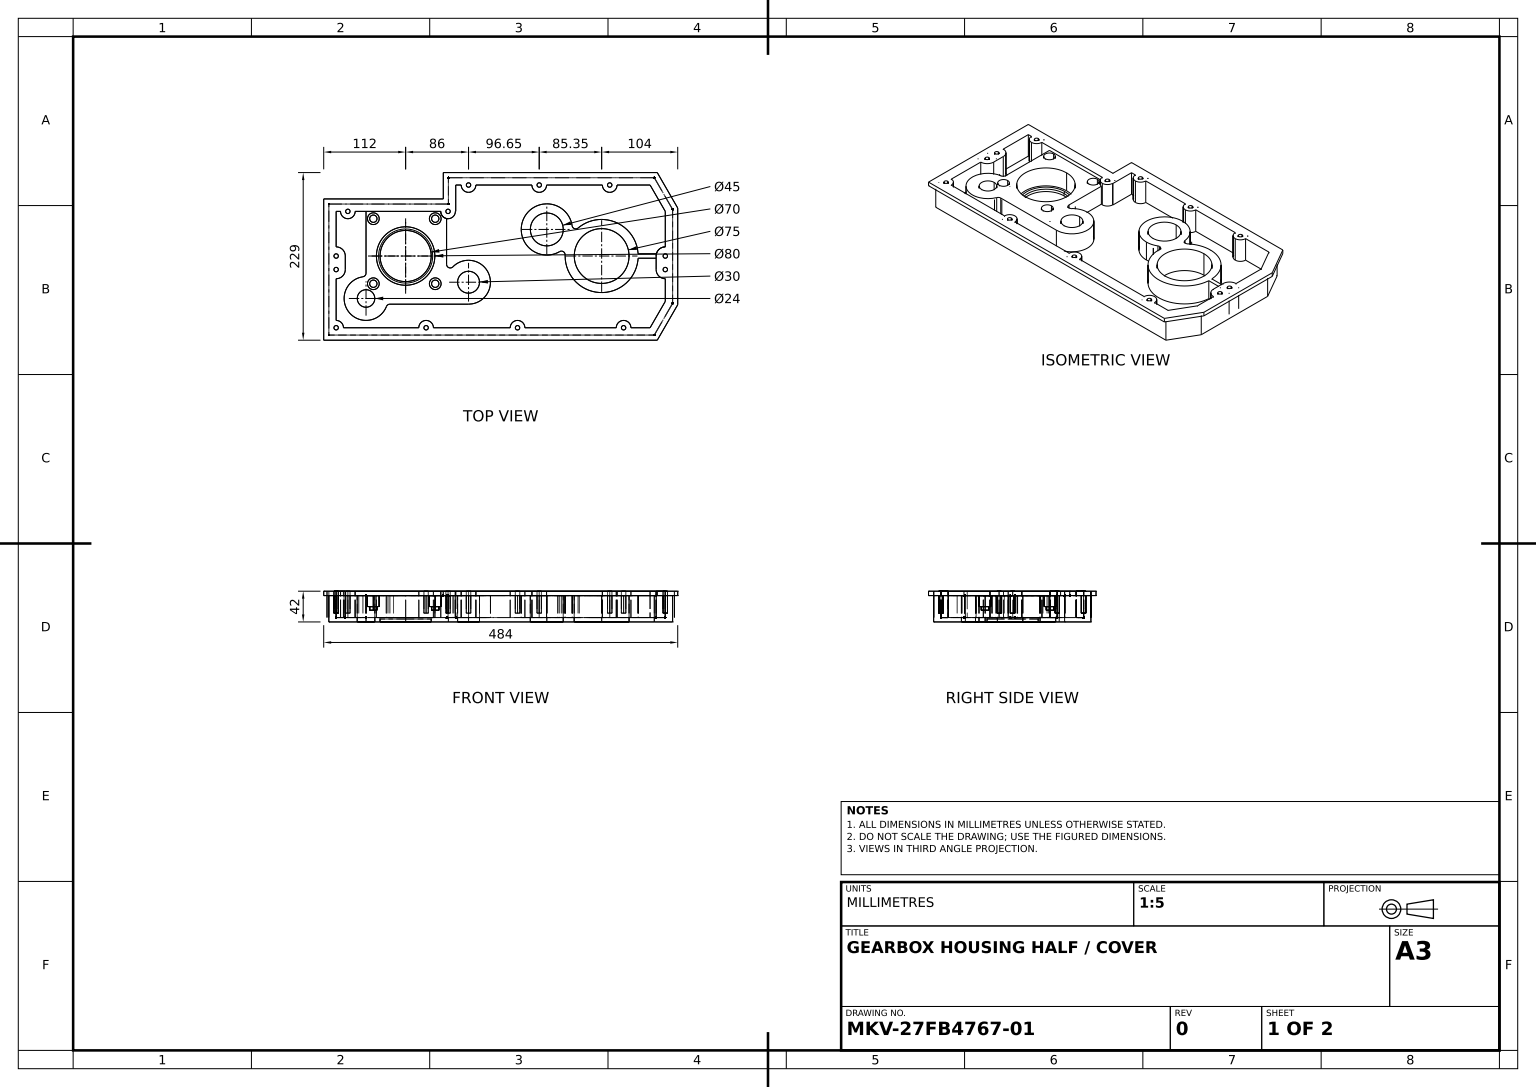
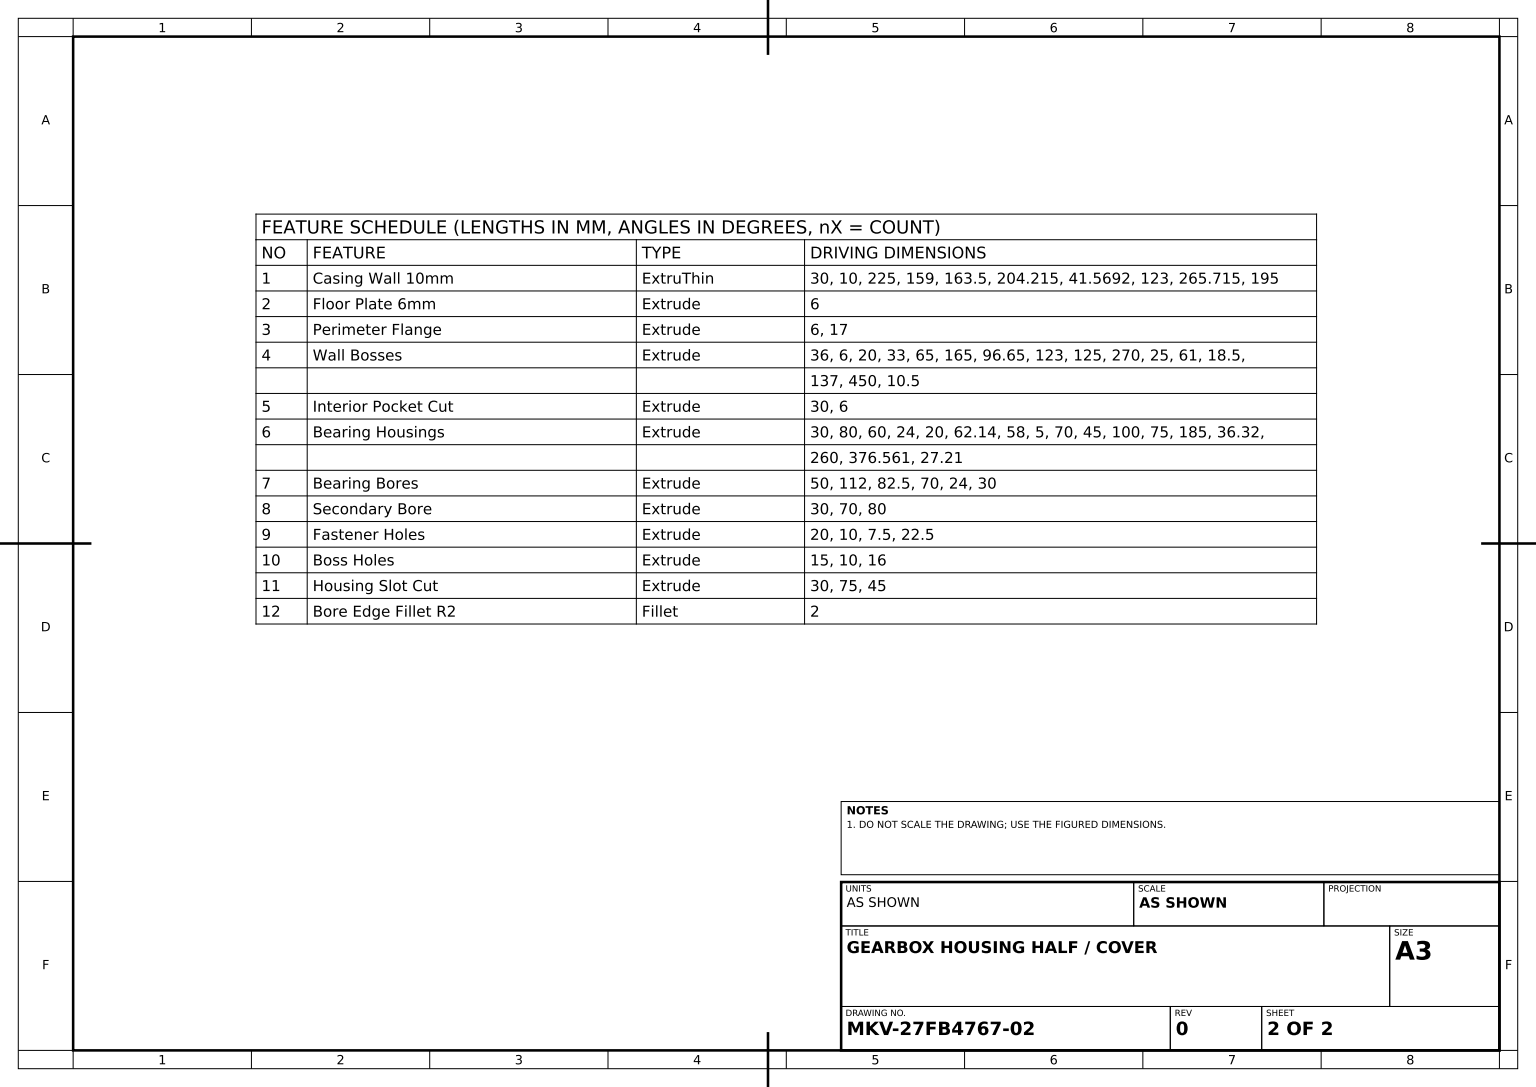
from build123d import *

# Parameters (mm, degrees)
CASING_WALL_10MM_DEPTH      = 30
FLOOR_PLATE_6MM_DEPTH       = 6
PERIMETER_FLANGE_DEPTH      = 6
WALL_BOSSES_DEPTH           = 36
INTERIOR_POCKET_SKETCH_R    = 3
INTERIOR_POCKET_CUT_DEPTH   = 30
BEARING_START               = 30
BEARING_HOUSINGS_SKETCH_R   = 12
BEARING_HOUSINGS_SKETCH_R_2 = 15
BEARING_HOUSINGS_SKETCH_R_3 = 40
BEARING_HOUSINGS_SKETCH_R_4 = 22.5
BEARING_HOUSINGS_SKETCH_R_5 = 37.5
BEARING_HOUSINGS_DEPTH      = 30
BEARING_BORES_SKETCH_R      = 35
BEARING_BORES_SKETCH_R_2    = 12
BEARING_BORES_SKETCH_R_3    = 15
BEARING_BORES_DEPTH         = 50
SECONDARY_BORE_SKETCH_R     = 40
SECONDARY_BORE_SKETCH_R_2   = 35
SECONDARY_BORE_DEPTH        = 30
FASTENER_HOLES_SKETCH_R     = 5
FASTENER_HOLES_DEPTH        = 20
BOSS_HOLES_SKETCH_R         = 8
BOSS_HOLES_SKETCH_R_2       = 5
BOSS_HOLES_DEPTH            = 15
HOUSING_SLOT_SKETCH_R       = 22.5
HOUSING_SLOT_SKETCH_R_2     = 37.5
HOUSING_SLOT_CUT_DEPTH      = 30
BORE_EDGE_FILLET_R2_R       = 2


with BuildPart() as part:
    # Casing Outline Sketch → Casing Wall 10mm (new body)
    with BuildSketch(Plane(origin=(0, 0, 0), x_dir=(1, 0, 0), z_dir=(0, 1, 0))):
        Polygon((235, 33.320508076), (235, 161.679491924), (209.988893001, 205), (-71.5, 205), (-71.5, 169), (-235, 169), (-235, -10), (209.988893001, -10), align=None)
        Polygon((225, 36), (225, 159), (204.215390309, 195), (-61.5, 195), (-61.5, 159), (-225, 159), (-225, 0), (204.215390309, 0), align=None, mode=Mode.SUBTRACT)
    extrude(amount=CASING_WALL_10MM_DEPTH)

    # Floor Plate Sketch → Floor Plate 6mm (add)
    with BuildSketch(Plane.XZ):
        Polygon((-235, 10), (-235, -169), (-71.5, -169), (-71.5, -205), (209.988893001, -205), (235, -161.679491924), (235, -33.320508076), (209.988893001, 10), align=None)
    extrude(amount=FLOOR_PLATE_6MM_DEPTH)

    # Perimeter Flange Sketch → Perimeter Flange (add)
    with BuildSketch(Plane(origin=(0, 30, 0), x_dir=(1, 0, 0), z_dir=(0, 1, 0))):
        Polygon((-242, 176), (-78.5, 176), (-78.5, 212), (214.030344885, 212), (242, 163.555136271), (242, 31.444863729), (214.030344885, -17), (-242, -17), align=None)
        Polygon((-225, 0), (-225, 159), (-61.5, 159), (-61.5, 195), (204.215390309, 195), (225, 159), (225, 36), (204.215390309, 0), align=None, mode=Mode.SUBTRACT)
    extrude(amount=PERIMETER_FLANGE_DEPTH)

    # Wall Bosses Sketch → Wall Bosses (add)
    with BuildSketch(Plane(origin=(0, 36, 0), x_dir=(1, 0, 0), z_dir=(0, 1, 0))):
        with BuildLine():
            ThreePointArc((-54, 195), (-44, 185), (-34, 195))
            Line((-34, 195), (-41, 195))
            ThreePointArc((-41, 195), (-44, 192), (-47, 195))
            Line((-47, 195), (-54, 195))
        make_face()
        with BuildLine():
            Line((-47, 195), (-41, 195))
            ThreePointArc((-41, 195), (-44, 198), (-47, 195))
        make_face()
        with BuildLine():
            ThreePointArc((-47, 195), (-44, 192), (-41, 195))
            Line((-41, 195), (-47, 195))
        make_face()
        with BuildLine():
            ThreePointArc((42.65, 195), (52.65, 185), (62.65, 195))
            Line((62.65, 195), (55.65, 195))
            ThreePointArc((55.65, 195), (52.65, 192), (49.65, 195))
            Line((49.65, 195), (42.65, 195))
        make_face()
        with BuildLine():
            Line((49.65, 195), (55.65, 195))
            ThreePointArc((55.65, 195), (52.65, 198), (49.65, 195))
        make_face()
        with BuildLine():
            ThreePointArc((49.65, 195), (52.65, 192), (55.65, 195))
            Line((55.65, 195), (49.65, 195))
        make_face()
        with BuildLine():
            ThreePointArc((139.030344885, 195), (149.030344885, 185), (159.030344885, 195))
            Line((159.030344885, 195), (152.030344885, 195))
            ThreePointArc((152.030344885, 195), (149.030344885, 192), (146.030344885, 195))
            Line((146.030344885, 195), (139.030344885, 195))
        make_face()
        with BuildLine():
            Line((146.030344885, 195), (152.030344885, 195))
            ThreePointArc((152.030344885, 195), (149.030344885, 198), (146.030344885, 195))
        make_face()
        with BuildLine():
            ThreePointArc((146.030344885, 195), (149.030344885, 192), (152.030344885, 195))
            Line((152.030344885, 195), (146.030344885, 195))
        make_face()
        with BuildLine():
            ThreePointArc((212.5, 79.5), (216.161165235, 70.661165235), (225, 67))
            Line((225, 67), (225, 76.5))
            ThreePointArc((225, 76.5), (222, 79.5), (225, 82.5))
            Line((225, 82.5), (225, 95))
            ThreePointArc((225, 95), (222, 98), (225, 101))
            Line((225, 101), (225, 110.5))
            ThreePointArc((225, 110.5), (216.161165235, 106.838834765), (212.5, 98))
            Line((212.5, 98), (212.5, 79.5))
        make_face()
        with BuildLine():
            Line((225, 101), (225, 95))
            ThreePointArc((225, 95), (227.121320344, 95.878679656), (228, 98))
            ThreePointArc((228, 98), (227.121320344, 100.121320344), (225, 101))
        make_face()
        with BuildLine():
            ThreePointArc((225, 101), (222, 98), (225, 95))
            Line((225, 95), (225, 101))
        make_face()
        with BuildLine():
            Line((225, 82.5), (225, 76.5))
            ThreePointArc((225, 76.5), (227.121320344, 77.378679656), (228, 79.5))
            ThreePointArc((228, 79.5), (227.121320344, 81.621320344), (225, 82.5))
        make_face()
        with BuildLine():
            ThreePointArc((225, 82.5), (222, 79.5), (225, 76.5))
            Line((225, 76.5), (225, 82.5))
        make_face()
        with BuildLine():
            Line((-212, 159), (-219, 159))
            ThreePointArc((-219, 159), (-209, 149), (-199, 159))
            Line((-199, 159), (-206, 159))
            ThreePointArc((-206, 159), (-209, 156), (-212, 159))
        make_face()
        with BuildLine():
            Line((-206, 159), (-212, 159))
            ThreePointArc((-212, 159), (-209, 156), (-206, 159))
        make_face()
        with BuildLine():
            ThreePointArc((-206, 159), (-209, 162), (-212, 159))
            Line((-212, 159), (-206, 159))
        make_face()
        with BuildLine():
            Line((-69, 159), (-75, 159))
            ThreePointArc((-75, 159), (-72, 156), (-69, 159))
        make_face()
        with BuildLine():
            ThreePointArc((-69, 159), (-72, 162), (-75, 159))
            Line((-75, 159), (-69, 159))
        make_face()
        with BuildLine():
            Line((-75, 159), (-82, 159))
            ThreePointArc((-82, 159), (-72, 149), (-62, 159))
            Line((-62, 159), (-69, 159))
            ThreePointArc((-69, 159), (-72, 156), (-75, 159))
        make_face()
        with BuildLine():
            Line((-225, 95), (-225, 101))
            ThreePointArc((-225, 101), (-228, 98), (-225, 95))
        make_face()
        with BuildLine():
            ThreePointArc((-222, 98), (-222.878679656, 100.121320344), (-225, 101))
            Line((-225, 101), (-225, 95))
            ThreePointArc((-225, 95), (-222.878679656, 95.878679656), (-222, 98))
        make_face()
        with BuildLine():
            Line((-225, 76.5), (-225, 82.5))
            ThreePointArc((-225, 82.5), (-228, 79.5), (-225, 76.5))
        make_face()
        with BuildLine():
            ThreePointArc((-222, 79.5), (-222.878679656, 81.621320344), (-225, 82.5))
            Line((-225, 82.5), (-225, 76.5))
            ThreePointArc((-225, 76.5), (-222.878679656, 77.378679656), (-222, 79.5))
        make_face()
        with BuildLine():
            ThreePointArc((-212.5, 98), (-216.161165235, 106.838834765), (-225, 110.5))
            Line((-225, 110.5), (-225, 101))
            ThreePointArc((-225, 101), (-222.878679656, 100.121320344), (-222, 98))
            ThreePointArc((-222, 98), (-222.878679656, 95.878679656), (-225, 95))
            Line((-225, 95), (-225, 82.5))
            ThreePointArc((-225, 82.5), (-222.878679656, 81.621320344), (-222, 79.5))
            ThreePointArc((-222, 79.5), (-222.878679656, 77.378679656), (-225, 76.5))
            Line((-225, 76.5), (-225, 67))
            ThreePointArc((-225, 67), (-216.161165235, 70.661165235), (-212.5, 79.5))
            Line((-212.5, 79.5), (-212.5, 98))
        make_face()
        with BuildLine():
            Line((-225, 0), (-225, 3))
            ThreePointArc((-225, 3), (-227.121320344, -2.121320344), (-222, 0))
            Line((-222, 0), (-225, 0))
        make_face()
        with BuildLine():
            ThreePointArc((-222, 0), (-222.878679656, 2.121320344), (-225, 3))
            Line((-225, 3), (-225, 0))
            Line((-225, 0), (-222, 0))
        make_face()
        with BuildLine():
            ThreePointArc((-215, 0), (-217.928932188, 7.071067812), (-225, 10))
            Line((-225, 10), (-225, 3))
            ThreePointArc((-225, 3), (-222.878679656, 2.121320344), (-222, 0))
            Line((-222, 0), (-215, 0))
        make_face()
        with BuildLine():
            Line((-99, 0), (-105, 0))
            ThreePointArc((-105, 0), (-102, -3), (-99, 0))
        make_face()
        with BuildLine():
            ThreePointArc((-99, 0), (-102, 3), (-105, 0))
            Line((-105, 0), (-99, 0))
        make_face()
        with BuildLine():
            ThreePointArc((-92, 0), (-102, 10), (-112, 0))
            Line((-112, 0), (-105, 0))
            ThreePointArc((-105, 0), (-102, 3), (-99, 0))
            Line((-99, 0), (-92, 0))
        make_face()
        with BuildLine():
            ThreePointArc((33, 0), (23, 10), (13, 0))
            Line((13, 0), (20, 0))
            ThreePointArc((20, 0), (23, 3), (26, 0))
            Line((26, 0), (33, 0))
        make_face()
        with BuildLine():
            Line((26, 0), (20, 0))
            ThreePointArc((20, 0), (23, -3), (26, 0))
        make_face()
        with BuildLine():
            ThreePointArc((26, 0), (23, 3), (20, 0))
            Line((20, 0), (26, 0))
        make_face()
        with BuildLine():
            ThreePointArc((178, 0), (168, 10), (158, 0))
            Line((158, 0), (165, 0))
            ThreePointArc((165, 0), (168, 3), (171, 0))
            Line((171, 0), (178, 0))
        make_face()
        with BuildLine():
            Line((171, 0), (165, 0))
            ThreePointArc((165, 0), (168, -3), (171, 0))
        make_face()
        with BuildLine():
            ThreePointArc((171, 0), (168, 3), (165, 0))
            Line((165, 0), (171, 0))
        make_face()
    extrude(amount=-WALL_BOSSES_DEPTH)

    # Interior Pocket Sketch → Interior Pocket Cut (cut)
    with BuildSketch(Plane(origin=(0, 36, 0), x_dir=(1, 0, 0), z_dir=(0, 1, 0))):
        with Locations(Location((-209, 159, 0), (0, 0, 270))):
            Circle(INTERIOR_POCKET_SKETCH_R)
        with Locations(Location((-72, 159, 0), (0, 0, 270))):
            Circle(INTERIOR_POCKET_SKETCH_R)
        with Locations(Location((-44, 195, 0), (0, 0, 270))):
            Circle(INTERIOR_POCKET_SKETCH_R)
        with Locations(Location((52.65, 195, 0), (0, 0, 270))):
            Circle(INTERIOR_POCKET_SKETCH_R)
        with Locations(Location((149.030344885, 195, 0), (0, 0, 270))):
            Circle(INTERIOR_POCKET_SKETCH_R)
        with Locations(Location((225, 98, 0), (0, 0, 270))):
            Circle(INTERIOR_POCKET_SKETCH_R)
        with Locations(Location((225, 79.5, 0), (0, 0, 270))):
            Circle(INTERIOR_POCKET_SKETCH_R)
        with Locations(Location((168, 0, 0), (0, 0, 270))):
            Circle(INTERIOR_POCKET_SKETCH_R)
        with Locations(Location((23, 0, 0), (0, 0, 270))):
            Circle(INTERIOR_POCKET_SKETCH_R)
        with Locations(Location((-225, 98, 0), (0, 0, 270))):
            Circle(INTERIOR_POCKET_SKETCH_R)
        with Locations(Location((-225, 79.5, 0), (0, 0, 270))):
            Circle(INTERIOR_POCKET_SKETCH_R)
        with Locations(Location((-225, 0, 0), (0, 0, 270))):
            Circle(INTERIOR_POCKET_SKETCH_R)
        with Locations(Location((-102, 0, 0), (0, 0, 270))):
            Circle(INTERIOR_POCKET_SKETCH_R)
    extrude(amount=-INTERIOR_POCKET_CUT_DEPTH, mode=Mode.SUBTRACT)

    # Bearing Housings Sketch → Bearing Housings (add)
    # profile 1 of 4: a face of its own
    with BuildSketch(Plane(origin=(0, 0, 0), x_dir=(1, 0, 0), z_dir=(0, 1, 0)).offset(BEARING_START)):
        with BuildLine():
            ThreePointArc((-65.428571429, 83.205626367), (-70.889822365, 82.075796929), (-74, 86.704897428))
            Line((-74, 86.704897428), (-74, 149.202041029))
            ThreePointArc((-74, 149.202041029), (-79.745966692, 152.67544468), (-82, 159))
            Line((-82, 159), (-184.14, 159))
            Line((-184.14, 159), (-184.14, 74.641016151))
            ThreePointArc((-184.14, 74.641016151), (-185.36035527, 71.367747798), (-188.425714286, 69.692299558))
            ThreePointArc((-188.425714286, 69.692299558), (-207.65417752, 21.36982406), (-156.214818474, 29.037142857))
            ThreePointArc((-156.214818474, 29.037142857), (-154.377027571, 31.341326318), (-151.560621553, 32.21))
            Line((-151.560621553, 32.21), (-44, 32.21))
            ThreePointArc((-44, 32.21), (-16.342552621, 73.831772864), (-65.428571429, 83.205626367))
        make_face()
        with Locations(Location((-184.14, 40, 0), (0, 0, 270))):
            Circle(BEARING_HOUSINGS_SKETCH_R, mode=Mode.SUBTRACT)
        with Locations(Location((-44, 62.21, 0), (0, 0, 270))):
            Circle(BEARING_HOUSINGS_SKETCH_R_2, mode=Mode.SUBTRACT)
        with Locations((-122, 98)):
            Circle(BEARING_HOUSINGS_SKETCH_R_3, mode=Mode.SUBTRACT)
    # profile 2 of 4: a face of its own
    with BuildSketch(Plane(origin=(0, 0, 0), x_dir=(1, 0, 0), z_dir=(0, 1, 0)).offset(BEARING_START)):
        with BuildLine():
            ThreePointArc((88.023723402, 99.540057585), (183.000978656, 76.20752607), (105.802940773, 136.253749844))
            ThreePointArc((105.802940773, 136.253749844), (100.806249829, 135.405547587), (97.635330494, 139.359234225))
            ThreePointArc((97.635330494, 139.359234225), (31.499314941, 149.574731751), (80.522833774, 104.022305426))
            ThreePointArc((80.522833774, 104.022305426), (85.590876722, 103.986137262), (88.023723402, 99.540057585))
        make_face()
        with Locations(Location((63, 134.32, 0), (0, 0, 270))):
            Circle(BEARING_HOUSINGS_SKETCH_R_4, mode=Mode.SUBTRACT)
        with Locations(Location((138, 98, 0), (0, 0, 270))):
            Circle(BEARING_HOUSINGS_SKETCH_R_5, mode=Mode.SUBTRACT)
    # profile 3 of 4: a face of its own
    with BuildSketch(Plane(origin=(0, 0, 0), x_dir=(1, 0, 0), z_dir=(0, 1, 0)).offset(BEARING_START)):
        with BuildLine():
            ThreePointArc((187.909918854, 101), (188, 98), (187.909918854, 95))
            Line((187.909918854, 95), (212.5, 95))
            Line((212.5, 95), (212.5, 98))
            ThreePointArc((212.5, 98), (212.591670867, 99.511081774), (212.8653389, 101))
            Line((212.8653389, 101), (187.909918854, 101))
        make_face()
    # profile 4 of 4: a face of its own
    with BuildSketch(Plane(origin=(0, 0, 0), x_dir=(1, 0, 0), z_dir=(0, 1, 0)).offset(BEARING_START)):
        with Locations((-122, 98)):
            Circle(BEARING_HOUSINGS_SKETCH_R_3)
    extrude(amount=-BEARING_HOUSINGS_DEPTH)

    # Bearing Bores Sketch → Bearing Bores (cut)
    with BuildSketch(Plane(origin=(0, 30, 0), x_dir=(1, 0, 0), z_dir=(0, 1, 0))):
        with Locations(Location((-130, 98, 0), (0, 0, 270))):
            Circle(BEARING_BORES_SKETCH_R)
        with Locations(Location((-184.14, 40, 0), (0, 0, 90))):
            Circle(BEARING_BORES_SKETCH_R_2)
        with Locations(Location((-44, 62.21, 0), (0, 0, 90))):
            Circle(BEARING_BORES_SKETCH_R_3)
    extrude(amount=-BEARING_BORES_DEPTH, mode=Mode.SUBTRACT)

    # Secondary Bore Sketch → Secondary Bore (cut)
    with BuildSketch(Plane(origin=(0, 30, 0), x_dir=(1, 0, 0), z_dir=(0, 1, 0))):
        with Locations(Location((-130, 98, 0), (0, 0, 270))):
            Circle(SECONDARY_BORE_SKETCH_R)
        with Locations(Location((-130, 98, 0), (0, 0, 270))):
            Circle(SECONDARY_BORE_SKETCH_R_2, mode=Mode.SUBTRACT)
    extrude(amount=-SECONDARY_BORE_DEPTH, mode=Mode.SUBTRACT)

    # Fastener Holes Sketch → Fastener Holes (cut)
    with BuildSketch(Plane(origin=(0, 30, 0), x_dir=(1, 0, 0), z_dir=(0, 1, 0))):
        with Locations(Location((-174.14, 149, 0), (0, 0, 270))):
            Circle(FASTENER_HOLES_SKETCH_R)
        with Locations(Location((-89.5, 149, 0), (0, 0, 270))):
            Circle(FASTENER_HOLES_SKETCH_R)
        with Locations(Location((-89.5, 60.155644371, 0), (0, 0, 270))):
            Circle(FASTENER_HOLES_SKETCH_R)
        with Locations(Location((-174.14, 60.155644371, 0), (0, 0, 270))):
            Circle(FASTENER_HOLES_SKETCH_R)
    extrude(amount=-FASTENER_HOLES_DEPTH, mode=Mode.SUBTRACT)

    # Boss Holes Sketch → Boss Holes (cut)
    # profile 1 of 4: a face of its own
    with BuildSketch(Plane(origin=(0, 30, 0), x_dir=(1, 0, 0), z_dir=(0, 1, 0))):
        with Locations(Location((-174.14, 149, 0), (0, 0, 270))):
            Circle(BOSS_HOLES_SKETCH_R)
        with Locations(Location((-174.14, 149, 0), (0, 0, 270))):
            Circle(BOSS_HOLES_SKETCH_R_2, mode=Mode.SUBTRACT)
    # profile 2 of 4: a face of its own
    with BuildSketch(Plane(origin=(0, 30, 0), x_dir=(1, 0, 0), z_dir=(0, 1, 0))):
        with Locations(Location((-89.5, 149, 0), (0, 0, 270))):
            Circle(BOSS_HOLES_SKETCH_R)
        with Locations(Location((-89.5, 149, 0), (0, 0, 270))):
            Circle(BOSS_HOLES_SKETCH_R_2, mode=Mode.SUBTRACT)
    # profile 3 of 4: a face of its own
    with BuildSketch(Plane(origin=(0, 30, 0), x_dir=(1, 0, 0), z_dir=(0, 1, 0))):
        with Locations(Location((-174.14, 60.155644371, 0), (0, 0, 270))):
            Circle(BOSS_HOLES_SKETCH_R)
        with Locations(Location((-174.14, 60.155644371, 0), (0, 0, 270))):
            Circle(BOSS_HOLES_SKETCH_R_2, mode=Mode.SUBTRACT)
    # profile 4 of 4: a face of its own
    with BuildSketch(Plane(origin=(0, 30, 0), x_dir=(1, 0, 0), z_dir=(0, 1, 0))):
        with Locations(Location((-89.5, 60.155644371, 0), (0, 0, 270))):
            Circle(BOSS_HOLES_SKETCH_R)
        with Locations(Location((-89.5, 60.155644371, 0), (0, 0, 270))):
            Circle(BOSS_HOLES_SKETCH_R_2, mode=Mode.SUBTRACT)
    extrude(amount=-BOSS_HOLES_DEPTH, mode=Mode.SUBTRACT)

    # Housing Slot Sketch → Housing Slot Cut (cut)
    with BuildSketch(Plane(origin=(0, 0, 0), x_dir=(1, 0, 0), z_dir=(0, 1, 0))):
        with Locations(Location((63, 134.32, 0), (0, 0, 90))):
            Circle(HOUSING_SLOT_SKETCH_R)
        with Locations(Location((138, 98, 0), (0, 0, 90))):
            Circle(HOUSING_SLOT_SKETCH_R_2)
    extrude(amount=-HOUSING_SLOT_CUT_DEPTH, mode=Mode.SUBTRACT)

    # Bore Edge Fillet R2
    bore_edge_fillet_r2_edges = [part.edges().sort_by_distance(p)[0] for p in [
        (-130, 0, -133),
    ]]
    fillet(bore_edge_fillet_r2_edges, radius=BORE_EDGE_FILLET_R2_R)


solid = part.part
